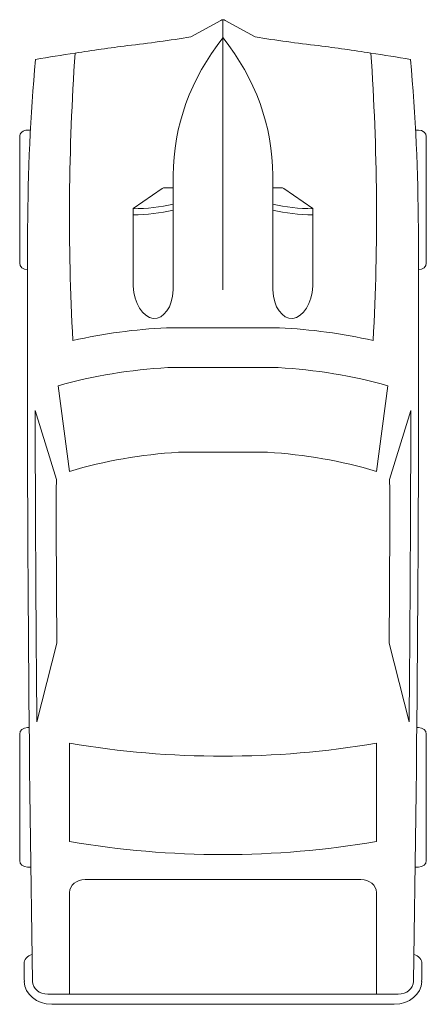
# Model space of a CAD drawing. Units: inches. Extents: x 5312 to 23584, y 2846 to 7447.
# Tile 12 of 12: x 23507 to 23584, y 6446 to 6635. Entities that reach past the tile are written whole.
import ezdxf

# ---------------------------------------------------------------- set-up
doc = ezdxf.new("R2010")
doc.units = ezdxf.units.IN
doc.layers.add('A-EQPM-VEHI', color=8, linetype='Continuous', lineweight=18)

# ---------------------------------------------------------------- blocks, each defined once
blk = doc.blocks.new('*U14')
for p, q in [((46.55, 38.89), (22.35, 38.89)), ((136.7, 38.89), (160.9, 38.89)), ((21.1, 37.41), (21.1, 36.83)), ((47.8, 37.39), (47.8, 37.41)), ((87.99, 31.87), (74.76, 35.92)), ((135.45, 37.07), (135.45, 37.41)), ((162.15, 37.41), (162.15, 36.77)), ((134.31, 35.6), (119.29, 31.78)), ((186.47, -33.5), (186.47, 33.5)), ((188.4, -32.76), (188.4, 32.76)), ((70.03, 31.54), (86.41, 29.35)), ((138.42, 29.35), (157.25, 29.35)), ((186.47, 29.35), (167.01, 29.35)), ((164.52, 26.39), (164.52, -26.39)), ((32.27, 11.63), (36.13, 17.17)), ((36.13, 17.17), (50.94, 17.17)), ((29.77, 9.51), (51.68, 9.51)), ((32.12, 9.51), (32.12, 11.15)), ((58.92, -10.77), (58.92, 10.77)), ((66.55, -10.53), (66.55, 10.53)), ((186.47, -10.53), (186.47, 10.53)), ((82.74, 8.5), (82.74, -8.5)), ((3.27, 6.13), (0.1, 0.41)), ((0, 0), (51.68, 0)), ((0.1, -0.41), (3.27, -6.13)), ((29.77, -9.51), (51.68, -9.51)), ((32.12, -9.51), (32.12, -11.15)), ((32.27, -11.63), (36.13, -17.17)), ((36.13, -17.17), (50.94, -17.17)), ((86.41, -29.35), (70.03, -31.54)), ((157.25, -29.35), (138.42, -29.35)), ((167.01, -29.35), (186.47, -29.35)), ((87.99, -31.87), (74.76, -35.92)), ((134.31, -35.6), (119.29, -31.78)), ((21.1, -37.41), (21.1, -36.83)), ((47.8, -37.39), (47.8, -37.41)), ((135.45, -37.07), (135.45, -37.41)), ((162.15, -37.41), (162.15, -36.77)), ((46.55, -38.89), (22.35, -38.89)), ((136.7, -38.89), (160.9, -38.89))]:
    blk.add_line(p, q)
for centre, major_axis, ratio, start_param, end_param in [((22.35, 37.41), (0, -1.48), 0.842304, 3.141593, 4.712389), ((46.55, 37.41), (0, 1.48), 0.842304, -1.570796, 0), ((136.7, 37.41), (0, -1.48), 0.842304, 3.141593, 4.712389), ((160.9, 37.41), (0, 1.48), 0.842304, -1.570796, 0), ((180.63, 35.84), (0, 2.22), 0.842304, -0.013017, 1.249894), ((64.48, -10556.36), (0, 10595.31), 0.842304, -0.013397, -0.013017), ((183.98, 32.76), (0, -5.25), 0.842304, 1.570796, 3.128196), ((266.03, -27.52), (0, 313.31), 0.842304, 1.367076, 1.39176), ((41.19, -490.86), (0, 528.23), 0.842304, 0.00281, 0.075598), ((64.48, -10555.62), (0, 10593.03), 0.842304, -0.013397, 0.002797), ((64.48, -10555.62), (0, -10591.55), 0.842304, 3.133765, 3.140441), ((183.98, 33.5), (0, -2.96), 0.842304, 1.570796, 3.128196), ((135.29, 5.39), (0, 81.77), 0.842304, 1.245306, 1.50788), ((95.79, -3666.35), (0, -3698.24), 0.842304, 3.134049, 3.144098), ((259.18, -27.52), (0, -305.3), 0.842304, 4.528606, 4.561838), ((37.47, -593.96), (0, -623.33), 0.842304, 3.096046, 3.200911), ((134.4, 5.39), (0, -89.78), 0.842304, 4.449482, 4.652344), ((149.6, 2.8), (0, -79.58), 0.842304, 4.372215, 4.640744), ((17.08, 0), (0, 147.02), 0.842304, 4.511394, 4.913384), ((35.91, 0), (0, 147.02), 0.842304, 4.511394, 4.913384), ((167.01, 26.39), (0, 2.96), 0.842304, 0, 1.570796), ((-204.49, 52.4), (0, -250.96), 0.842304, 1.385369, 1.434372), ((13.04, 17.01), (0, 27.42), 0.842304, 4.435146, 4.718221), ((14.2, 17.01), (0, 27.42), 0.842304, 4.435146, 4.718221), ((50.79, 13.34), (6.34, -0.36), 0.603834, -1.395552, 1.581315), ((32.75, 11.15), (0, 0.74), 0.842304, 0.879714, 1.570796), ((29.77, -46.66), (0, 56.17), 0.842304, 0, 0.590319), ((0.62, 0), (0, -0.74), 0.842304, 4.131459, 5.293319), ((29.77, 46.66), (0, 56.17), 0.842304, 2.551274, 3.141593), ((-204.49, -52.4), (0, 250.96), 0.842304, -1.434372, -1.385369), ((149.6, -2.8), (0, -79.58), 0.842304, -1.499151, -1.230623), ((32.75, -11.15), (0, -0.74), 0.842304, 4.712389, 5.403472), ((13.04, -17.01), (0, -27.42), 0.842304, 1.564964, 1.848039), ((14.2, -17.01), (0, -27.42), 0.842304, 1.564964, 1.848039), ((134.4, -5.39), (0, -89.78), 0.842304, -1.510751, -1.307889), ((135.29, -5.39), (0, -81.77), 0.842304, -1.50788, -1.245306), ((259.18, 27.52), (0, 305.3), 0.842304, 1.721348, 1.754579), ((167.01, -26.39), (0, -2.96), 0.842304, 4.712389, 6.283185), ((266.03, 27.52), (0, 313.31), 0.842304, 1.749832, 1.774517), ((37.47, 593.96), (0, -623.33), 0.842304, -0.059319, 0.045547), ((95.79, 3666.35), (0, -3698.24), 0.842304, -0.002505, 0.007544), ((183.98, -33.5), (0, 2.96), 0.842304, 3.15499, 4.712389), ((183.98, -32.76), (0, -5.25), 0.842304, 0.013397, 1.570796), ((64.48, 10555.62), (0, -10591.55), 0.842304, 0.001152, 0.007828), ((41.19, 490.86), (0, -528.23), 0.842304, -0.075598, -0.00281), ((22.35, -37.41), (0, 1.48), 0.842304, 1.570796, 3.141593), ((64.48, 10555.62), (0, 10593.03), 0.842304, 3.138796, 3.15499), ((46.55, -37.41), (0, -1.48), 0.842304, 0, 1.570796), ((136.7, -37.41), (0, -1.48), 0.842304, -1.570796, 0), ((160.9, -37.41), (0, 1.48), 0.842304, 3.141593, 4.712389), ((180.63, -35.84), (0, -2.22), 0.842304, -1.249894, 0.013017), ((64.48, 10556.36), (0, 10595.31), 0.842304, 3.15461, 3.15499)]:
    blk.add_ellipse(centre, major_axis=major_axis, ratio=ratio, start_param=start_param, end_param=end_param)
at = {"extrusion": (0, 0, -1)}
blk.add_ellipse((50.79, -13.34), major_axis=(6.34, 0.36), ratio=0.603834, start_param=-1.395552, end_param=1.581315, dxfattribs=at)

msp = doc.modelspace()

# ---------------------------------------------------------------- block references
at = {"layer": 'A-EQPM-VEHI', "rotation": 270}
msp.add_blockref('*U14', (23545.57, 6634.705), dxfattribs=at)

doc.saveas('drawing.dxf')
